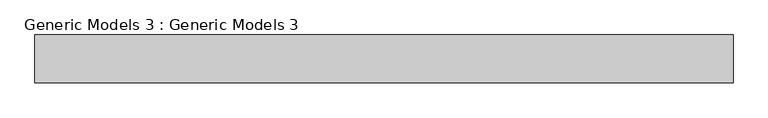
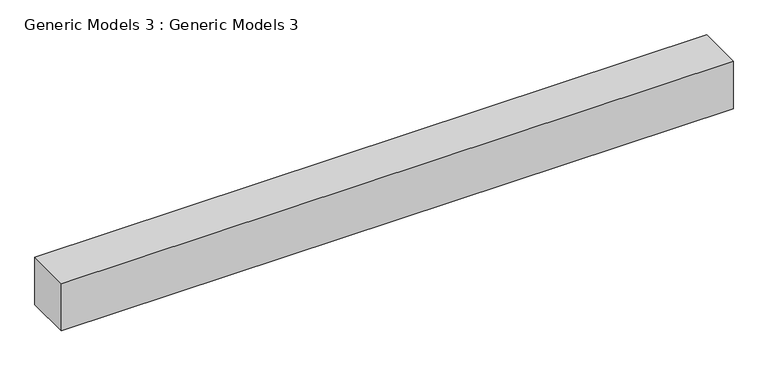
"""IFC4 building model written with IfcOpenShell, lengths in millimetres: proxy geometry, Generic Models 3 : Generic Models 3."""

from ifc_helpers import new_model, si_unit, frame, origin, place, context, project, spatial, polyline, outline, extrude, source, transform, mapped, element, save


def generic_models_3_generic_models_3_4fdafdf2(model_context):
    return source(origin(), model_context, "Body", "SweptSolid", [
        extrude(outline(polyline([(4815.8764826, -3746.0004242), (4815.8764826, -4114.1934365), (-562.0138036, -4114.1934365), (-562.0138036, -3746.0004242), (4815.8764826, -3746.0004242)])), frame((0.0, 0.0, 2739.850832), z_axis=(0.0, 0.0, 1.0), x_axis=(1.0, 0.0, 0.0)), (0.0, 0.0, 1.0), 399.7658161),
    ])


if __name__ == "__main__":
    model = new_model("IFC4")
    model_context = context("Model", 3, world=origin())
    ifc_project = project(units=[si_unit("LENGTHUNIT", "METRE", prefix="MILLI")], contexts=[model_context])
    site = spatial("IfcSite", under=ifc_project)
    building = spatial("IfcBuilding", under=site)
    placement = place(None, origin())
    generic_models_3_generic_models_3_shape = generic_models_3_generic_models_3_4fdafdf2(model_context)
    element("IfcBuildingElementProxy", 1, Name="Generic Models 3 : Generic Models 3", ObjectType="Generic Models 3 : Generic Models 3", at=placement, inside=building, context=model_context, shape_type="MappedRepresentation", body=[
        mapped(generic_models_3_generic_models_3_shape, transform((0.0, 0.0, 0.0), x_axis=(1.0, 0.0, 0.0), y_axis=(0.0, 1.0, 0.0), z_axis=(0.0, 0.0, 1.0))),
    ])
    save(model, "model.ifc")
